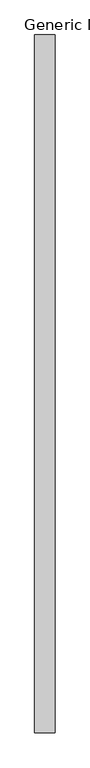
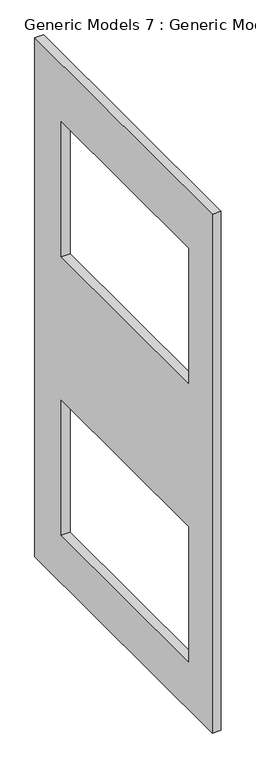
"""IFC4 building model written with IfcOpenShell, lengths in millimetres: proxy geometry, Generic Models 7 : Generic Models 7."""

from ifc_helpers import new_model, si_unit, frame, origin, place, context, project, spatial, polyline, outline, extrude, source, transform, mapped, element, save


def generic_models_7_generic_models_7_fc47f9bb(model_context):
    return source(origin(), model_context, "Body", "SweptSolid", [
        extrude(outline(polyline([(4078.7605753, 6280.076449), (4078.7605753, 31.676449), (573.5605753, 31.676449), (573.5605753, 6280.076449), (4078.7605753, 6280.076449)]), holes=[polyline([(3554.2974325, 5588.0), (1039.6974325, 5588.0), (1039.6974325, 3962.4), (3554.2974325, 3962.4), (3554.2974325, 5588.0)]), polyline([(3554.2974325, 2235.2), (1039.6974325, 2235.2), (1039.6974325, 609.6), (3554.2974325, 609.6), (3554.2974325, 2235.2)])]), frame((-6788.929089, 0.0, 0.0), z_axis=(1.0, 0.0, 0.0), x_axis=(0.0, 1.0, 0.0)), (0.0, 0.0, 1.0), 101.6),
    ])


if __name__ == "__main__":
    model = new_model("IFC4")
    model_context = context("Model", 3, world=origin())
    ifc_project = project(units=[si_unit("LENGTHUNIT", "METRE", prefix="MILLI")], contexts=[model_context])
    site = spatial("IfcSite", under=ifc_project)
    building = spatial("IfcBuilding", under=site)
    placement = place(None, origin())
    generic_models_7_generic_models_7_shape = generic_models_7_generic_models_7_fc47f9bb(model_context)
    element("IfcBuildingElementProxy", 1, Name="Generic Models 7 : Generic Models 7", ObjectType="Generic Models 7 : Generic Models 7", at=placement, inside=building, context=model_context, shape_type="MappedRepresentation", body=[
        mapped(generic_models_7_generic_models_7_shape, transform((0.0, 0.0, 0.0), x_axis=(1.0, 0.0, 0.0), y_axis=(0.0, 1.0, 0.0), z_axis=(0.0, 0.0, 1.0))),
    ])
    save(model, "model.ifc")

# Revit data of these elements
# Element 1 (IfcBuildingElementProxy, "Generic Models 7 : Generic Models 7")
#   Materials on its faces: "Wood Planks"
# Materials
#   "Wood Planks": class "Wood", colour RGB 129 72 39, transparency 0, Description = "Physical material.", Cost = 0
